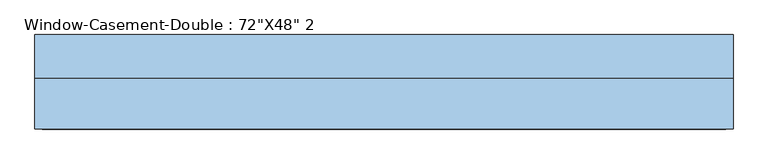
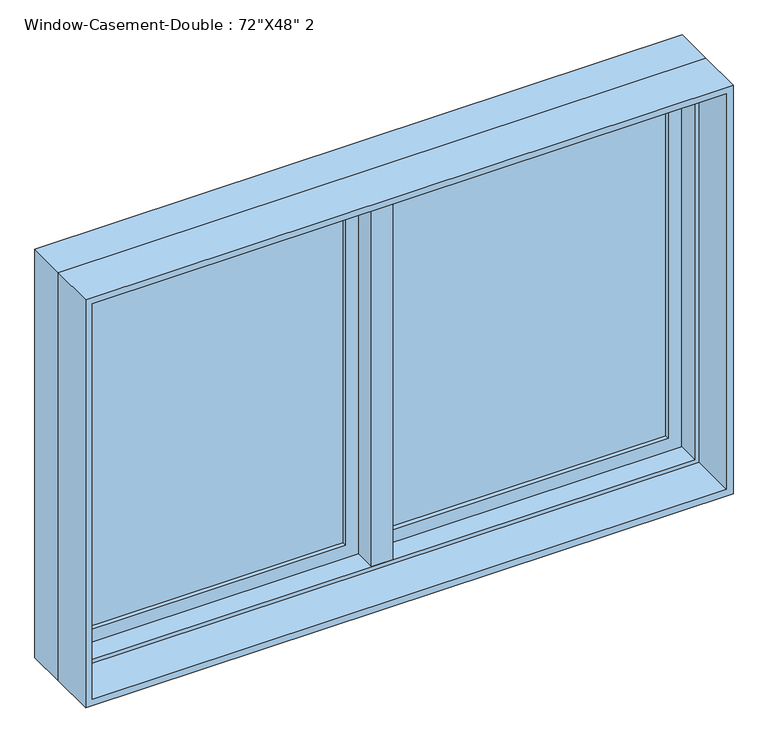
"""IFC4 building model written with IfcOpenShell, lengths in millimetres: window geometry."""

from ifc_helpers import new_model, si_unit, frame, origin, place, context, project, spatial, polyline, outline, extrude, faceted_brep, source, transform, mapped, element, save


def window_bf2f09a8(model_context):
    return source(origin(), model_context, "Body", "SolidModel", [
        faceted_brep([(9.525, 133.35, 2120.9), (-9.525, 133.35, 2120.9), (-9.525, 82.55, 2120.9), (9.525, 82.55, 2120.9), (9.525, 133.35, 927.1), (9.525, 82.55, 927.1), (-9.525, 82.55, 927.1), (-9.525, 133.35, 927.1), (-9.525, 82.55, 946.15), (-9.525, 82.55, 2101.85), (-30.1625, 82.55, 946.15), (-30.1625, 82.55, 2101.85), (-30.1625, 19.05, 946.15), (-30.1625, 19.05, 2101.85), (30.1625, 19.05, 946.15), (30.1625, 19.05, 2101.85), (30.1625, 82.55, 946.15), (30.1625, 82.55, 2101.85), (9.525, 82.55, 946.15), (9.525, 82.55, 2101.85)], [[[0, 1, 2, 3]], [[4, 5, 6, 7]], [[1, 0, 4, 7]], [[2, 1, 7, 6, 8, 9]], [[9, 8, 10, 11]], [[11, 10, 12, 13]], [[13, 12, 14, 15]], [[15, 14, 16, 17]], [[17, 16, 18, 19]], [[0, 3, 19, 18, 5, 4]], [[18, 8, 6, 5]], [[9, 19, 3, 2]], [[8, 18, 16, 14, 12, 10]], [[19, 9, 11, 13, 15, 17]]]),
        extrude(outline(polyline([(-66.675, 114.3), (-66.675, 107.95), (-844.55, 107.95), (-844.55, 114.3), (-66.675, 114.3)])), frame((0.0, 0.0, 984.25), z_axis=(0.0, 0.0, 1.0), x_axis=(1.0, 0.0, 0.0)), (0.0, 0.0, 1.0), 1079.5),
        extrude(outline(polyline([(-844.55, 95.25), (-844.55, 101.6), (-66.675, 101.6), (-66.675, 95.25), (-844.55, 95.25)])), frame((0.0, 0.0, 984.25), z_axis=(0.0, 0.0, 1.0), x_axis=(1.0, 0.0, 0.0)), (0.0, 0.0, 1.0), 1079.5),
        extrude(outline(polyline([(844.55, 114.3), (844.55, 107.95), (66.675, 107.95), (66.675, 114.3), (844.55, 114.3)])), frame((0.0, 0.0, 984.25), z_axis=(0.0, 0.0, 1.0), x_axis=(1.0, 0.0, 0.0)), (0.0, 0.0, 1.0), 1079.5),
        extrude(outline(polyline([(66.675, 95.25), (66.675, 101.6), (844.55, 101.6), (844.55, 95.25), (66.675, 95.25)])), frame((0.0, 0.0, 984.25), z_axis=(0.0, 0.0, 1.0), x_axis=(1.0, 0.0, 0.0)), (0.0, 0.0, 1.0), 1079.5),
        extrude(outline(polyline([(2120.9, -901.7), (927.1, -901.7), (927.1, -9.525), (2120.9, -9.525), (2120.9, -901.7)]), holes=[polyline([(2063.75, -66.675), (984.25, -66.675), (984.25, -844.55), (2063.75, -844.55), (2063.75, -66.675)])]), frame((0.0, 82.55, 0.0), z_axis=(0.0, 1.0, 0.0), x_axis=(0.0, 0.0, 1.0)), (0.0, 0.0, 1.0), 44.45),
        extrude(outline(polyline([(927.1, 901.7), (2120.9, 901.7), (2120.9, 9.525), (927.1, 9.525), (927.1, 901.7)]), holes=[polyline([(984.25, 66.675), (2063.75, 66.675), (2063.75, 844.55), (984.25, 844.55), (984.25, 66.675)])]), frame((0.0, 82.55, 0.0), z_axis=(0.0, 1.0, 0.0), x_axis=(0.0, 0.0, 1.0)), (0.0, 0.0, 1.0), 44.45),
        extrude(outline(polyline([(2133.6, -914.4), (914.4, -914.4), (914.4, 914.4), (2133.6, 914.4), (2133.6, -914.4)]), holes=[polyline([(2114.55, 895.35), (933.45, 895.35), (933.45, -895.35), (2114.55, -895.35), (2114.55, 895.35)])]), frame((0.0, -114.3, 0.0), z_axis=(0.0, 1.0, 0.0), x_axis=(0.0, 0.0, 1.0)), (0.0, 0.0, 1.0), 133.35),
        faceted_brep([(882.65, 82.55, 2101.85), (882.65, 19.05, 2101.85), (-882.65, 19.05, 2101.85), (-882.65, 82.55, 2101.85), (901.7, 133.35, 2120.9), (901.7, 82.55, 2120.9), (-901.7, 82.55, 2120.9), (-901.7, 133.35, 2120.9), (914.4, 19.05, 2133.6), (914.4, 133.35, 2133.6), (-914.4, 133.35, 2133.6), (-914.4, 19.05, 2133.6), (-882.65, 19.05, 946.15), (-882.65, 82.55, 946.15), (-901.7, 82.55, 927.1), (-901.7, 133.35, 927.1), (-914.4, 133.35, 914.4), (-914.4, 19.05, 914.4), (882.65, 19.05, 946.15), (882.65, 82.55, 946.15), (901.7, 82.55, 927.1), (901.7, 133.35, 927.1), (914.4, 133.35, 914.4), (914.4, 19.05, 914.4)], [[[0, 1, 2, 3]], [[4, 5, 6, 7]], [[8, 9, 10, 11]], [[3, 2, 12, 13]], [[7, 6, 14, 15]], [[11, 10, 16, 17]], [[13, 12, 18, 19]], [[15, 14, 20, 21]], [[17, 16, 22, 23]], [[11, 17, 23, 8], [1, 18, 12, 2]], [[19, 18, 1, 0]], [[5, 20, 14, 6], [3, 13, 19, 0]], [[21, 20, 5, 4]], [[23, 22, 9, 8]], [[9, 22, 16, 10], [7, 15, 21, 4]]]),
    ])


if __name__ == "__main__":
    model = new_model("IFC4")
    model_context = context("Model", 3, world=origin())
    ifc_project = project(units=[si_unit("LENGTHUNIT", "METRE", prefix="MILLI")], contexts=[model_context])
    site = spatial("IfcSite", under=ifc_project)
    building = spatial("IfcBuilding", under=site)
    placement = place(None, origin())
    window_shape = window_bf2f09a8(model_context)
    element("IfcWindow", 1, ObjectType="Window-Casement-Double : 72\"X48\" 2", at=placement, inside=building, context=model_context, shape_type="MappedRepresentation", body=[
        mapped(window_shape, transform((0.0, 0.0, 0.0), x_axis=(1.0, 0.0, 0.0), y_axis=(0.0, 1.0, 0.0), z_axis=(0.0, 0.0, 1.0))),
    ])
    save(model, "model.ifc")

# Revit data of these elements
# Type "Window-Casement-Double : 72\"X48\" 2"
#   Type Mark = "26"
#   Fire Rating = "0.5h"
#   Assembly Code = "B2020100"
#   Analytic Construction = "Double glazing - domestic"
#   Frame Extension [instance default] = 0' - 0 1/4"
#   Window Inset [instance default] = 0' - 0"
#   Wall Thickness [instance default] = 0' - 6"
#   Interior Wall Closure [instance default] = 0' - 2 1/4"
#   Half Width = 3' - 0"
#   Visual Light Transmittance = 0.81
#   Thermal Resistance (R) = 1.8146 (h·ft²·°F)/BTU
#   Solar Heat Gain Coefficient = 0.76
#   Rough Width = 6' - 0 1/2"
#   Rough Height = 4' - 0 1/2"
#   Height = 4' - 0"
#   Heat Transfer Coefficient (U) = 0.5511 BTU/(h·ft²·°F)
#   Exterior Wall Closure [instance default] = 0' - 1 1/4"
#   Extension Jamb [instance default] = 0' - 2 1/4"
#   Default Sill Height = 3' - 0"
#   Width = 6' - 0"
#   Muntin Visibility = yes
#   Interior Trim Visibility [instance default] = yes
#   Exterior Trim Visibility [instance default] = yes
#   Extension Jamb Visibility [instance default] = yes
#   Interior Trim Material = Wood - Stained
#   Muntin Pattern = Muntin Pattern_2x2 : Muntin Pattern_2x2
#   Interior Trim = Trim-Window-Interior-Flat : Picture Frame
#   Interior Frame Material = Wood - Stained
#   Glass Panel Material = Glass
#   Exterior Trim Material = Clad - White
#   Exterior Trim = Trim-Window-Exterior-Flat : with Sill
#   Exterior Frame Material = Clad - White
#   Wall Closure = (empty or 0)
# Element 1 (IfcWindow, "Window-Casement-Double : 72\"X48\" 2")
#   Wall Thickness = 0' - 9"
#   Extension Jamb = 0' - 5 1/4"
#   Materials on its faces: "Wood - Stained", "Glass", "Clad - White"
# Materials
#   "Wood - Stained": class "Wood", colour RGB 224 178 126, transparency 0, Cost = 0
#   "Glass": class "Glass", colour RGB 0 128 192, transparency 0.75, Description = "Soda Lime Glass", Cost = 0
#   "Clad - White": class "Wood", colour RGB 242 242 238, transparency 0, Cost = 0
